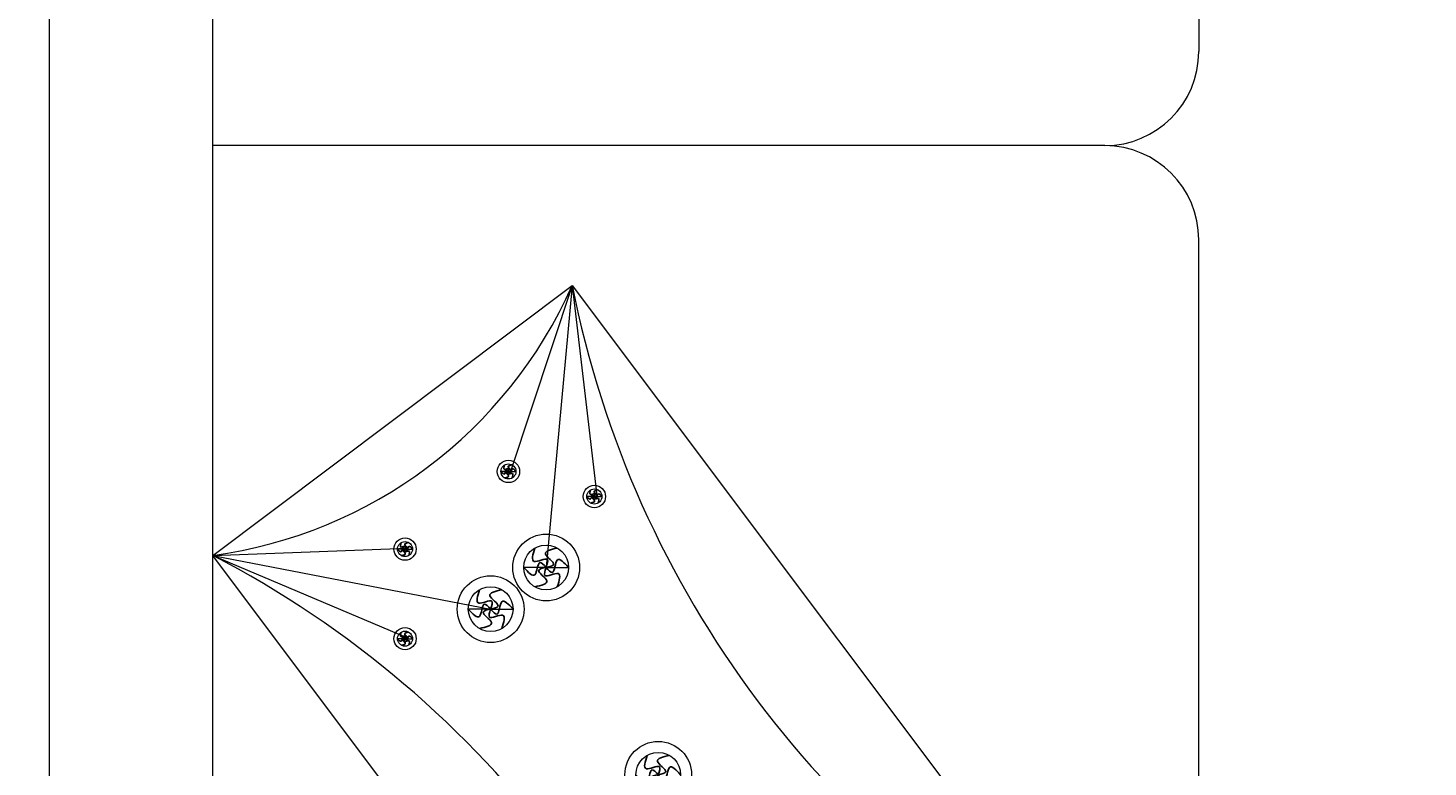
# Model space of a CAD drawing. Units: inches. Extents: x -61 to 1599, y -1316 to 257.
# Tile 130 of 204: x 388 to 418, y -122 to -106. Entities that reach past the tile are written whole.
import ezdxf

# ---------------------------------------------------------------- set-up
doc = ezdxf.new("R2010")
doc.units = ezdxf.units.IN
doc.header["$MEASUREMENT"] = 0
doc.layers.add('A-ANNO-DIMS', color=2, linetype='Continuous', lineweight=18)
doc.layers.add('FURNITURE', color=83, linetype='Continuous', lineweight=18)
doc.layers.add('FUR', color=83, linetype='Continuous')
doc.styles.get("Standard").update_dxf_attribs({"font": 'arial.ttf'})
doc.dimstyles.get("Standard").update_dxf_attribs({"dimtxt": 0.18, "dimasz": 0.18, "dimexe": 0.18, "dimexo": 0.0625, "dimgap": 0.09, "dimtad": 0, "dimtih": 1, "dimtoh": 1, "dimdec": 0, "dimzin": 0, "dimdsep": 46, "dimlunit": 3, "dimtxsty": 'Standard', "dimcen": 0.09, "dimadec": 0, "dimazin": 0, "dimtfac": 1, "dimtdec": 0, "dimtofl": 0, "dimtmove": 0, "dimatfit": 3, "dimfxl": 1, "dimtolj": 1, "dimtzin": 0, "dimarcsym": 0})

# ---------------------------------------------------------------- blocks, each defined once
blk = doc.blocks.new('*U160')
at = {"layer": 'FUR'}
blk.add_open_spline([(0.005, 0.08), (-0.03, 0.048), (-0.098, -0.015), (0.075, -0.018), (0.024, -0.063), (0.005, -0.08)], degree=3, knots=[0, 0, 0, 0, 0.0954578, 0.1898773, 0.2470677, 0.2470677, 0.2470677, 0.2470677], dxfattribs=at)
blk = doc.blocks.new('*U161')
at = {"layer": 'FUR', "transparency": 16777216}
for p, rotation in [((222.173, -79.977), 60), ((222.178, -80.056), 120), ((222.25, -80.092), 180), ((222.312, -79.968), 300), ((222.317, -80.048), 240)]:
    blk.add_blockref('*U160', p, dxfattribs=dict(at, rotation=rotation))
blk.add_blockref('*U160', (222.24, -79.932), dxfattribs=at)
blk = doc.blocks.new('*U172')
at = {"layer": 'FUR'}
blk.add_open_spline([(0.005, 0.08), (-0.03, 0.048), (-0.098, -0.015), (0.075, -0.018), (0.024, -0.063), (0.005, -0.08)], degree=3, knots=[0, 0, 0, 0, 0.0954578, 0.1898773, 0.2470677, 0.2470677, 0.2470677, 0.2470677], dxfattribs=at)
blk = doc.blocks.new('*U173')
at = {"layer": 'FUR', "transparency": 16777216}
for p, rotation in [((222.173, -79.977), 60), ((222.178, -80.056), 120), ((222.25, -80.092), 180), ((222.312, -79.968), 300), ((222.317, -80.048), 240)]:
    blk.add_blockref('*U172', p, dxfattribs=dict(at, rotation=rotation))
blk.add_blockref('*U172', (222.24, -79.932), dxfattribs=at)
blk = doc.blocks.new('*U184')
at = {"layer": 'FUR'}
blk.add_open_spline([(0.015, 0.238), (-0.088, 0.143), (-0.292, -0.045), (0.224, -0.053), (0.072, -0.187), (0.015, -0.238)], degree=3, knots=[0, 0, 0, 0, 0.2846533, 0.5662105, 0.736751, 0.736751, 0.736751, 0.736751], dxfattribs=at)
blk = doc.blocks.new('*U159')
at = {"layer": 'FUR', "transparency": 16777216}
blk.add_blockref('*U184', (662.716, -238.357), dxfattribs=at)
for p, rotation in [((662.929, -238.463), 300), ((662.517, -238.489), 60), ((662.531, -238.727), 120), ((662.944, -238.702), 240), ((662.745, -238.833), 180)]:
    blk.add_blockref('*U184', p, dxfattribs=dict(at, rotation=rotation))
blk = doc.blocks.new('*U174')
at = {"layer": 'FUR'}
blk.add_open_spline([(0.005, 0.08), (-0.03, 0.048), (-0.098, -0.015), (0.075, -0.018), (0.024, -0.063), (0.005, -0.08)], degree=3, knots=[0, 0, 0, 0, 0.0954578, 0.1898773, 0.2470677, 0.2470677, 0.2470677, 0.2470677], dxfattribs=at)
blk = doc.blocks.new('*U175')
at = {"layer": 'FUR', "transparency": 16777216}
for p, rotation in [((222.173, -79.977), 60), ((222.178, -80.056), 120), ((222.25, -80.092), 180), ((222.312, -79.968), 300), ((222.317, -80.048), 240)]:
    blk.add_blockref('*U174', p, dxfattribs=dict(at, rotation=rotation))
blk.add_blockref('*U174', (222.24, -79.932), dxfattribs=at)
blk = doc.blocks.new('*U168')
at = {"layer": 'FUR'}
blk.add_open_spline([(0.015, 0.238), (-0.088, 0.143), (-0.292, -0.045), (0.224, -0.053), (0.072, -0.187), (0.015, -0.238)], degree=3, knots=[0, 0, 0, 0, 0.2846533, 0.5662105, 0.736751, 0.736751, 0.736751, 0.736751], dxfattribs=at)
blk = doc.blocks.new('*U169')
at = {"layer": 'FUR', "transparency": 16777216}
blk.add_blockref('*U168', (662.716, -238.357), dxfattribs=at)
for p, rotation in [((662.929, -238.463), 300), ((662.517, -238.489), 60), ((662.531, -238.727), 120), ((662.944, -238.702), 240), ((662.745, -238.833), 180)]:
    blk.add_blockref('*U168', p, dxfattribs=dict(at, rotation=rotation))
blk = doc.blocks.new('*U176')
at = {"layer": 'FUR'}
blk.add_open_spline([(0.005, 0.08), (-0.03, 0.048), (-0.098, -0.015), (0.075, -0.018), (0.024, -0.063), (0.005, -0.08)], degree=3, knots=[0, 0, 0, 0, 0.0954578, 0.1898773, 0.2470677, 0.2470677, 0.2470677, 0.2470677], dxfattribs=at)
blk = doc.blocks.new('*U177')
at = {"layer": 'FUR', "transparency": 16777216}
for p, rotation in [((222.173, -79.977), 60), ((222.178, -80.056), 120), ((222.25, -80.092), 180), ((222.312, -79.968), 300), ((222.317, -80.048), 240)]:
    blk.add_blockref('*U176', p, dxfattribs=dict(at, rotation=rotation))
blk.add_blockref('*U176', (222.24, -79.932), dxfattribs=at)
blk = doc.blocks.new('*U170')
at = {"layer": 'FUR'}
blk.add_open_spline([(0.015, 0.238), (-0.088, 0.143), (-0.292, -0.045), (0.224, -0.053), (0.072, -0.187), (0.015, -0.238)], degree=3, knots=[0, 0, 0, 0, 0.2846533, 0.5662105, 0.736751, 0.736751, 0.736751, 0.736751], dxfattribs=at)
blk = doc.blocks.new('*U171')
at = {"layer": 'FUR', "transparency": 16777216}
blk.add_blockref('*U170', (662.716, -238.357), dxfattribs=at)
for p, rotation in [((662.929, -238.463), 300), ((662.517, -238.489), 60), ((662.531, -238.727), 120), ((662.944, -238.702), 240), ((662.745, -238.833), 180)]:
    blk.add_blockref('*U170', p, dxfattribs=dict(at, rotation=rotation))
blk = doc.blocks.new('SOFA-LOVESEAT')
for p, q in [((3.47, 8), (3.47, 52)), ((24.442, 52), (24.442, 32)), ((22.442, 30), (3.47, 30)), ((22.442, 30), (22.442, 30)), ((24.442, 8), (24.442, 28)), ((11.116, 27.026), (9.811, 23.092)), ((11.116, 27.026), (10.561, 21.032)), ((11.116, 27.026), (11.639, 22.56)), ((9.759, 23.073), (9.599, 23.073)), ((9.759, 23.073), (9.918, 23.073)), ((11.587, 22.541), (11.427, 22.541)), ((11.587, 22.541), (11.747, 22.541)), ((3.47, 21.288), (7.612, 21.442)), ((3.47, 21.288), (9.381, 20.146)), ((3.47, 21.288), (7.612, 19.538)), ((7.56, 21.423), (7.4, 21.423)), ((7.56, 21.423), (7.719, 21.423)), ((10.561, 21.032), (10.084, 21.032)), ((10.561, 21.032), (11.037, 21.032)), ((9.381, 20.146), (8.904, 20.146)), ((9.381, 20.146), (9.857, 20.146)), ((7.56, 19.518), (7.4, 19.518)), ((7.56, 19.518), (7.719, 19.518))]:
    blk.add_line(p, q)
blk.add_lwpolyline([(26, 6), (26, 2, -0.414214), (24, 0), (2, 0, -0.414214), (0, 2), (0, 58, -0.414213), (2, 60), (24, 60, -0.414214), (26, 58), (26, 54)], format="xyb")
blk.add_lwpolyline([(11.116, 27.026), (22.422, 11.961), (14.776, 6.223), (3.47, 21.288)], close=True)
for centre, radius in [((9.759, 23.073), 0.238), ((9.759, 23.073), 0.16), ((11.587, 22.541), 0.238), ((11.587, 22.541), 0.16), ((10.561, 21.032), 0.71), ((7.56, 21.423), 0.238), ((7.56, 21.423), 0.16), ((10.561, 21.032), 0.476), ((9.381, 20.146), 0.71), ((9.381, 20.146), 0.476), ((7.56, 19.518), 0.238), ((7.56, 19.518), 0.16), ((12.946, 16.624), 0.71), ((12.946, 16.624), 0.476)]:
    blk.add_circle(centre, radius)
for centre, radius, start, end in [((22.442, 32), 2, 270, 0), ((22.442, 28), 2, 0, 90), ((2.147, 31.014), 9.816, 277.747, 336.0258), ((32.433, 31.248), 21.731, 191.2044, 242.5684), ((-6.541, 2), 21.731, 11.2044, 62.5684)]:
    blk.add_arc(centre, radius, start, end)
at = {"rotation": 90}
for name, p in [('*U175', (-70.254, -199.172)), ('*U177', (-68.425, -199.704)), ('*U173', (-72.453, -200.822)), ('*U169', (-228.034, -641.698)), ('*U159', (-229.214, -642.584)), ('*U161', (-72.453, -202.727)), ('*U171', (-225.649, -646.106))]:
    blk.add_blockref(name, p, dxfattribs=at)
blk = doc.blocks.new('*D703')
at = {"layer": 'A-ANNO-DIMS', "color": 0, "lineweight": -2, "transparency": 16777216}
for p, q in [((372.32, -616.882), (372.32, 257.457)), ((372.5, 257.277), (413.7, 257.277)), ((455.653, 257.277), (414.453, 257.277)), ((455.833, -616.882), (455.833, 257.457))]:
    blk.add_line(p, q, dxfattribs=at)
at = {"layer": 'A-ANNO-DIMS', "color": 0, "transparency": 16777216}
for points in [[(372.5, 257.307), (372.5, 257.247), (372.32, 257.277)], [(455.653, 257.307), (455.653, 257.247), (455.833, 257.277)]]:
    blk.add_solid(points, dxfattribs=at)
at = {"layer": 'DEFPOINTS', "color": 0, "transparency": 16777216}
for p in [(455.833, 257.277), (372.32, -616.945), (455.833, -616.945)]:
    blk.add_point(p, dxfattribs=at)
at = {"layer": 'A-ANNO-DIMS', "color": 0, "transparency": 16777216, "insert": (414.076, 257.277), "char_height": 0.18, "attachment_point": 5}
blk.add_mtext('\\A1;83.51', dxfattribs=at)

msp = doc.modelspace()

# ---------------------------------------------------------------- block references
at = {"layer": 'FURNITURE'}
msp.add_blockref('SOFA-LOVESEAT', (388.9518, -138.383), dxfattribs=at)

# ---------------------------------------------------------------- dimensions: what is measured, and where the dimension line sits
at = {"layer": 'A-ANNO-DIMS'}
dim = msp.add_linear_dim(base=(455.8327, 257.2771), p1=(372.3201, -616.9446), p2=(455.8327, -616.9446), dimstyle='Standard', override={"dimdec": 2, "dimlfac": 1, "dimrnd": 0, "dimzin": 0, "dimdsep": 46, "dimlunit": 2}, dxfattribs=at)
dim.commit()
dim.dimension.update_dxf_attribs({"geometry": '*D703', "text_midpoint": (414.0764, 257.2771)})

doc.saveas('drawing.dxf')
